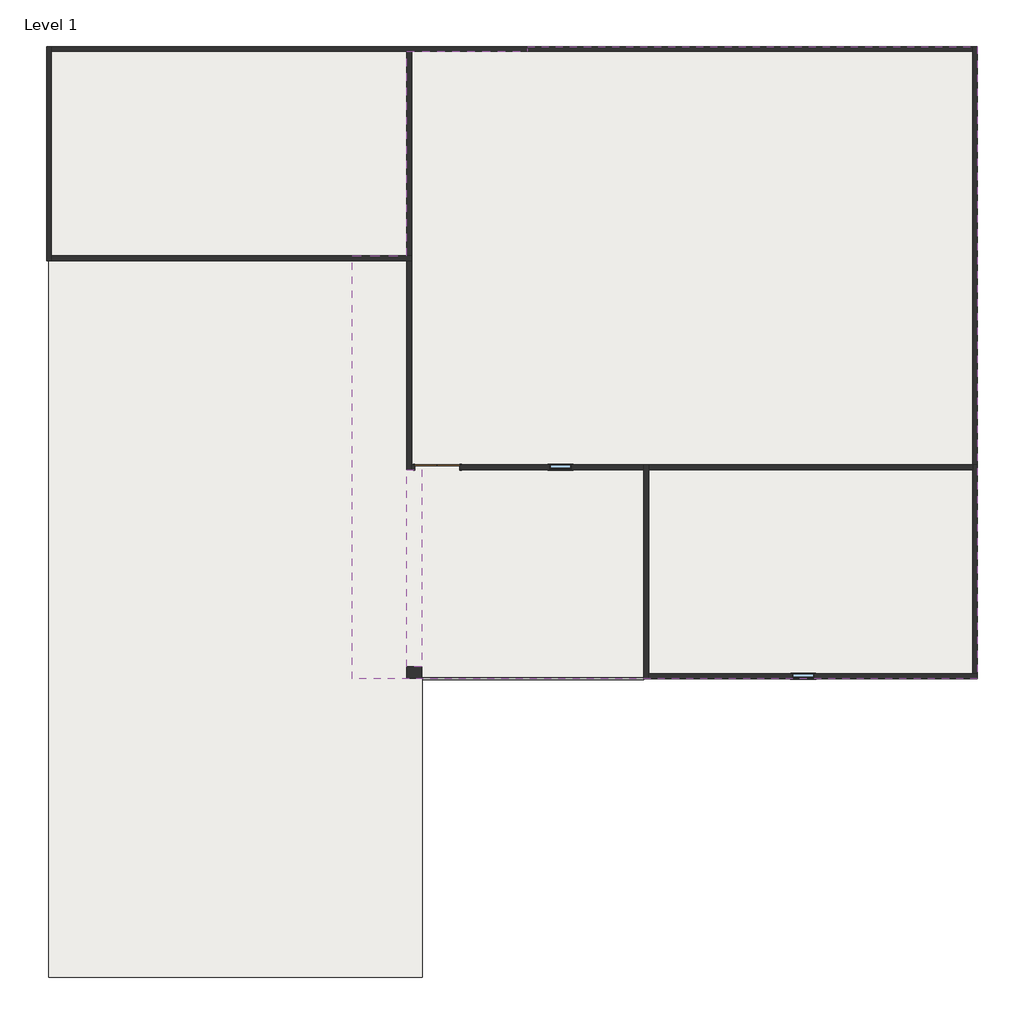
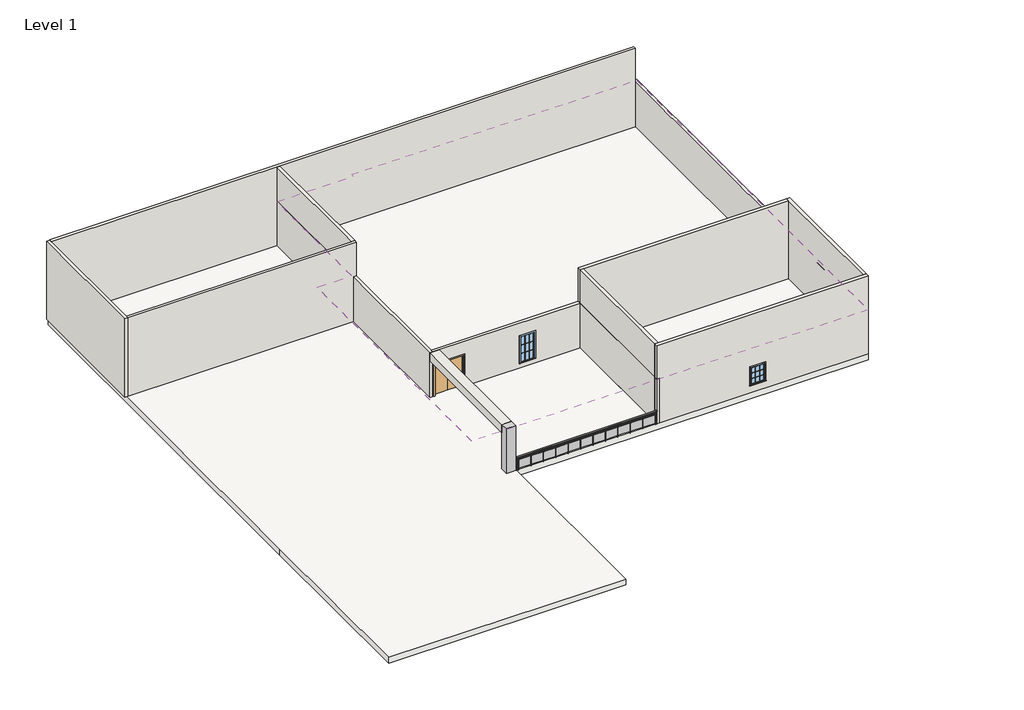
# One storey, incomplete: 13 walls, 2 windows, 1 column, 1 covering, 1 door, 1 railing, 1 slab.
"""IFC4 building model written with IfcOpenShell, lengths in millimetres."""

from ifc_helpers import new_model, si_unit, point, frame, origin, place, context, project, spatial, polyline, ellipse_curve, trimmed, outline, extrude, faceted_brep, transform, mapped, element, save
from ifc_brep_helpers import plane_surface, extruded_surface, advanced_brep
from components import m_rectangular_column_475_x_610mm_d36e7488, door_db0c0681, walls_1_walls_1_bd393664, window_ddc5d35f, window_0c844ac8

model = new_model("IFC4")

# Units and contexts
model_context = context("Model", 3, world=origin())
ifc_project = project(units=[si_unit("LENGTHUNIT", "METRE", prefix="MILLI")], contexts=[model_context])

# Site, building, storey
site = spatial("IfcSite", under=ifc_project)
building = spatial("IfcBuilding", under=site)
storey = spatial("IfcBuildingStorey", under=building, Name="Level 1", Elevation=3048.0)

# Column
placement = place(None, origin())
m_rectangular_column_475_x_610mm_shape = m_rectangular_column_475_x_610mm_d36e7488(model_context)
element("IfcColumn", 1, ObjectType="M_Rectangular Column : 475 x 610mm", at=placement, inside=storey, context=model_context, shape_type="MappedRepresentation", body=[
    mapped(m_rectangular_column_475_x_610mm_shape, transform((-2824.5479903, -9080.6874979, 0.0), x_axis=(1.0, 0.0, 0.0), y_axis=(0.0, 1.0, 0.0), z_axis=(0.0, 0.0, 1.0))),
])

# Covering
element("IfcCovering", 2, ObjectType="600 x 1200mm grid", at=placement, inside=storey, context=model_context, shape_type="SweptSolid", body=[
    extrude(outline(polyline([(-5354.6982739, -9333.0874979), (-5354.6982739, 7935.7125021), (-3125.3625081, 7935.7125021), (-3125.3625081, 16270.1125021), (1808.1017261, 16270.1125021), (1808.1017261, 16470.1125021), (20161.6374919, 16470.1125021), (20161.6374919, -9333.0874979), (-5354.6982739, -9333.0874979)]), holes=[polyline([(-4506.4859174, -9133.0874979), (6313.9140826, -9133.0874979), (6313.9140826, -7913.8874979), (-4506.4859174, -7913.8874979), (-4506.4859174, -9133.0874979)]), polyline([(-3051.6674392, 6921.3125021), (-4506.4859174, 6921.3125021), (-4506.4859174, -598.6874979), (-3051.6674392, -598.6874979), (-3051.6674392, 6921.3125021)])]), frame((0.0, 0.0, 6045.2), z_axis=(0.0, 0.0, 1.0), x_axis=(1.0, 0.0, 0.0)), (0.0, 0.0, 1.0), 52.0),
    extrude(outline(polyline([(-3473.1102813, -8081.6812121), (-3473.1102813, -8996.0812121), (-3549.3102813, -8996.0812121), (-3549.3102813, -8081.6812121), (-3473.1102813, -8081.6812121)])), frame((0.0, 0.0, 6045.2), z_axis=(0.0, 0.0, 1.0), x_axis=(1.0, 0.0, 0.0)), (0.0, 0.0, 1.0), 52.0),
    extrude(outline(polyline([(-2711.1102813, -8081.6812121), (-2711.1102813, -8996.0812121), (-2787.3102813, -8996.0812121), (-2787.3102813, -8081.6812121), (-2711.1102813, -8081.6812121)])), frame((0.0, 0.0, 6045.2), z_axis=(0.0, 0.0, 1.0), x_axis=(1.0, 0.0, 0.0)), (0.0, 0.0, 1.0), 52.0),
    extrude(outline(polyline([(-1771.3102813, -8081.6812121), (-1771.3102813, -8996.0812121), (-1847.5102813, -8996.0812121), (-1847.5102813, -8081.6812121), (-1771.3102813, -8081.6812121)])), frame((0.0, 0.0, 6045.2), z_axis=(0.0, 0.0, 1.0), x_axis=(1.0, 0.0, 0.0)), (0.0, 0.0, 1.0), 52.0),
    extrude(outline(polyline([(-856.9102813, -8081.6812121), (-856.9102813, -8996.0812121), (-933.1102813, -8996.0812121), (-933.1102813, -8081.6812121), (-856.9102813, -8081.6812121)])), frame((0.0, 0.0, 6045.2), z_axis=(0.0, 0.0, 1.0), x_axis=(1.0, 0.0, 0.0)), (0.0, 0.0, 1.0), 52.0),
    extrude(outline(polyline([(209.8897187, -8081.6812121), (209.8897187, -8996.0812121), (133.6897187, -8996.0812121), (133.6897187, -8081.6812121), (209.8897187, -8081.6812121)])), frame((0.0, 0.0, 6045.2), z_axis=(0.0, 0.0, 1.0), x_axis=(1.0, 0.0, 0.0)), (0.0, 0.0, 1.0), 52.0),
    extrude(outline(polyline([(1276.6897187, -8081.6812121), (1276.6897187, -8996.0812121), (1200.4897187, -8996.0812121), (1200.4897187, -8081.6812121), (1276.6897187, -8081.6812121)])), frame((0.0, 0.0, 6045.2), z_axis=(0.0, 0.0, 1.0), x_axis=(1.0, 0.0, 0.0)), (0.0, 0.0, 1.0), 52.0),
    extrude(outline(polyline([(2648.2897187, -8081.6812121), (2648.2897187, -8996.0812121), (2572.0897187, -8996.0812121), (2572.0897187, -8081.6812121), (2648.2897187, -8081.6812121)])), frame((0.0, 0.0, 6045.2), z_axis=(0.0, 0.0, 1.0), x_axis=(1.0, 0.0, 0.0)), (0.0, 0.0, 1.0), 52.0),
    extrude(outline(polyline([(4019.8897187, -8081.6812121), (4019.8897187, -8996.0812121), (3943.6897187, -8996.0812121), (3943.6897187, -8081.6812121), (4019.8897187, -8081.6812121)])), frame((0.0, 0.0, 6045.2), z_axis=(0.0, 0.0, 1.0), x_axis=(1.0, 0.0, 0.0)), (0.0, 0.0, 1.0), 52.0),
    extrude(outline(polyline([(5239.0897187, -8081.6812121), (5239.0897187, -8996.0812121), (5162.8897187, -8996.0812121), (5162.8897187, -8081.6812121), (5239.0897187, -8081.6812121)])), frame((0.0, 0.0, 6045.2), z_axis=(0.0, 0.0, 1.0), x_axis=(1.0, 0.0, 0.0)), (0.0, 0.0, 1.0), 52.0),
    extrude(outline(polyline([(-3153.2674392, 3237.4377462), (-3153.2674392, 2932.6377462), (-4423.2674392, 2932.6377462), (-4423.2674392, 3237.4377462), (-3153.2674392, 3237.4377462)])), frame((0.0, 0.0, 6045.2), z_axis=(0.0, 0.0, 1.0), x_axis=(1.0, 0.0, 0.0)), (0.0, 0.0, 1.0), 52.0),
    extrude(outline(polyline([(-3153.2674392, 5523.4377462), (-3153.2674392, 5218.6377462), (-4423.2674392, 5218.6377462), (-4423.2674392, 5523.4377462), (-3153.2674392, 5523.4377462)])), frame((0.0, 0.0, 6045.2), z_axis=(0.0, 0.0, 1.0), x_axis=(1.0, 0.0, 0.0)), (0.0, 0.0, 1.0), 52.0),
    extrude(outline(polyline([(-3153.2674392, 951.4377462), (-3153.2674392, 646.6377462), (-4423.2674392, 646.6377462), (-4423.2674392, 951.4377462), (-3153.2674392, 951.4377462)])), frame((0.0, 0.0, 6045.2), z_axis=(0.0, 0.0, 1.0), x_axis=(1.0, 0.0, 0.0)), (0.0, 0.0, 1.0), 52.0),
])

# Door
door_shape = door_db0c0681(model_context)
element("IfcDoor", 3, ObjectType="Door-Double-Flush_Panel : 72\" x 84\"", at=placement, inside=storey, context=model_context, shape_type="MappedRepresentation", body=[
    mapped(door_shape, transform((-1883.9625081, -698.6874979, 3048.0), x_axis=(1.0, 0.0, 0.0), y_axis=(0.0, 1.0, 0.0), z_axis=(0.0, 0.0, 1.0))),
])

# Railing
element("IfcRailing", 4, ObjectType="Glass Panel - Bottom Fill", at=placement, inside=storey, context=model_context, shape_type="SolidModel", body=[
    advanced_brep(
    [(-2473.5625081, -9293.6967328, 3948.0), (-2473.5625081, -9373.6967328, 3948.0), (6550.4374919, -9293.6967328, 3948.0), (6550.4374919, -9373.6967328, 3948.0)],
    [
        (0, 1, ellipse_curve(frame((-2473.5625081, -9333.6967328, 3948.0), z_axis=(-1.0, 0.0, 0.0), x_axis=(0.0, -1.0, 0.0)), 40.0, 30.0)),
        (1, 0, ellipse_curve(frame((-2473.5625081, -9333.6967328, 3948.0), z_axis=(-1.0, 0.0, 0.0), x_axis=(0.0, -1.0, 0.0)), 40.0, 30.0)),
        (2, 3, ellipse_curve(frame((6550.4374919, -9333.6967328, 3948.0), z_axis=(1.0, 0.0, 0.0), x_axis=(0.0, -1.0, 0.0)), 40.0, 30.0)),
        (3, 2, ellipse_curve(frame((6550.4374919, -9333.6967328, 3948.0), z_axis=(1.0, 0.0, 0.0), x_axis=(0.0, -1.0, 0.0)), 40.0, 30.0)),
        (1, 3),
        (2, 0),
    ],
    [
        plane_surface(frame((-2473.5625081, -9333.6967328, 3948.0), z_axis=(-1.0, 0.0, 0.0), x_axis=(0.0, 1.0, 0.0))),
        plane_surface(frame((6550.4374919, -9333.6967328, 3948.0), z_axis=(1.0, 0.0, 0.0), x_axis=(0.0, 1.0, 0.0))),
        extruded_surface(trimmed(ellipse_curve(frame((6550.4374919, -9333.6967328, 3948.0), z_axis=(-1.0, 0.0, 0.0), x_axis=(0.0, -1.0, 0.0)), 40.0, 30.0), [point((6550.4374919, -9373.6967328, 3948.0))], [point((6550.4374919, -9293.6967328, 3948.0))], True, "CARTESIAN"), (-9024.0, 0.0, 0.0), 9024.0),
        extruded_surface(trimmed(ellipse_curve(frame((6550.4374919, -9333.6967328, 3948.0), z_axis=(-1.0, 0.0, 0.0), x_axis=(0.0, -1.0, 0.0)), 40.0, 30.0), [point((6550.4374919, -9293.6967328, 3948.0))], [point((6550.4374919, -9373.6967328, 3948.0))], True, "CARTESIAN"), (-9024.0, 0.0, 0.0), 9024.0),
    ],
    [
        (0, [[1, 2]]),
        (1, [[3, 4]]),
        (2, [[-2, 5, -3, 6]]),
        (3, [[-1, -6, -4, -5]]),
    ],
),
    extrude(outline(polyline([(-2473.5625081, -9343.0874979), (-2473.5625081, -9323.0874979), (6550.4374919, -9323.0874979), (6550.4374919, -9343.0874979), (-2473.5625081, -9343.0874979)])), frame((0.0, 0.0, 3828.0), z_axis=(0.0, 0.0, 1.0), x_axis=(1.0, 0.0, 0.0)), (0.0, 0.0, 1.0), 20.0),
    extrude(outline(polyline([(-2473.5625081, -9343.0874979), (-2473.5625081, -9323.0874979), (6550.4374919, -9323.0874979), (6550.4374919, -9343.0874979), (-2473.5625081, -9343.0874979)])), frame((0.0, 0.0, 3728.0), z_axis=(0.0, 0.0, 1.0), x_axis=(1.0, 0.0, 0.0)), (0.0, 0.0, 1.0), 20.0),
    extrude(outline(polyline([(6432.4374919, -9308.0874979), (6444.4374919, -9308.0874979), (6444.4374919, -9358.0874979), (6432.4374919, -9358.0874979), (6432.4374919, -9308.0874979)])), frame((0.0, 0.0, 3048.0), z_axis=(0.0, 0.0, 1.0), x_axis=(1.0, 0.0, 0.0)), (0.0, 0.0, 1.0), 869.8465326),
    extrude(outline(polyline([(5638.4374919, -9334.812308), (6438.4374919, -9334.812308), (6438.4374919, -9339.812308), (5638.4374919, -9339.812308), (5638.4374919, -9334.812308)])), frame((0.0, 0.0, 3148.0), z_axis=(0.0, 0.0, 1.0), x_axis=(1.0, 0.0, 0.0)), (0.0, 0.0, 1.0), 580.0),
    extrude(outline(polyline([(5632.4374919, -9308.0874979), (5644.4374919, -9308.0874979), (5644.4374919, -9358.0874979), (5632.4374919, -9358.0874979), (5632.4374919, -9308.0874979)])), frame((0.0, 0.0, 3048.0), z_axis=(0.0, 0.0, 1.0), x_axis=(1.0, 0.0, 0.0)), (0.0, 0.0, 1.0), 869.8465326),
    extrude(outline(polyline([(4838.4374919, -9334.812308), (5638.4374919, -9334.812308), (5638.4374919, -9339.812308), (4838.4374919, -9339.812308), (4838.4374919, -9334.812308)])), frame((0.0, 0.0, 3148.0), z_axis=(0.0, 0.0, 1.0), x_axis=(1.0, 0.0, 0.0)), (0.0, 0.0, 1.0), 580.0),
    extrude(outline(polyline([(4832.4374919, -9308.0874979), (4844.4374919, -9308.0874979), (4844.4374919, -9358.0874979), (4832.4374919, -9358.0874979), (4832.4374919, -9308.0874979)])), frame((0.0, 0.0, 3048.0), z_axis=(0.0, 0.0, 1.0), x_axis=(1.0, 0.0, 0.0)), (0.0, 0.0, 1.0), 869.8465326),
    extrude(outline(polyline([(4038.4374919, -9334.812308), (4838.4374919, -9334.812308), (4838.4374919, -9339.812308), (4038.4374919, -9339.812308), (4038.4374919, -9334.812308)])), frame((0.0, 0.0, 3148.0), z_axis=(0.0, 0.0, 1.0), x_axis=(1.0, 0.0, 0.0)), (0.0, 0.0, 1.0), 580.0),
    extrude(outline(polyline([(4032.4374919, -9308.0874979), (4044.4374919, -9308.0874979), (4044.4374919, -9358.0874979), (4032.4374919, -9358.0874979), (4032.4374919, -9308.0874979)])), frame((0.0, 0.0, 3048.0), z_axis=(0.0, 0.0, 1.0), x_axis=(1.0, 0.0, 0.0)), (0.0, 0.0, 1.0), 869.8465326),
    extrude(outline(polyline([(3238.4374919, -9334.812308), (4038.4374919, -9334.812308), (4038.4374919, -9339.812308), (3238.4374919, -9339.812308), (3238.4374919, -9334.812308)])), frame((0.0, 0.0, 3148.0), z_axis=(0.0, 0.0, 1.0), x_axis=(1.0, 0.0, 0.0)), (0.0, 0.0, 1.0), 580.0),
    extrude(outline(polyline([(3232.4374919, -9308.0874979), (3244.4374919, -9308.0874979), (3244.4374919, -9358.0874979), (3232.4374919, -9358.0874979), (3232.4374919, -9308.0874979)])), frame((0.0, 0.0, 3048.0), z_axis=(0.0, 0.0, 1.0), x_axis=(1.0, 0.0, 0.0)), (0.0, 0.0, 1.0), 869.8465326),
    extrude(outline(polyline([(2438.4374919, -9334.812308), (3238.4374919, -9334.812308), (3238.4374919, -9339.812308), (2438.4374919, -9339.812308), (2438.4374919, -9334.812308)])), frame((0.0, 0.0, 3148.0), z_axis=(0.0, 0.0, 1.0), x_axis=(1.0, 0.0, 0.0)), (0.0, 0.0, 1.0), 580.0),
    extrude(outline(polyline([(2432.4374919, -9308.0874979), (2444.4374919, -9308.0874979), (2444.4374919, -9358.0874979), (2432.4374919, -9358.0874979), (2432.4374919, -9308.0874979)])), frame((0.0, 0.0, 3048.0), z_axis=(0.0, 0.0, 1.0), x_axis=(1.0, 0.0, 0.0)), (0.0, 0.0, 1.0), 869.8465326),
    extrude(outline(polyline([(1638.4374919, -9334.812308), (2438.4374919, -9334.812308), (2438.4374919, -9339.812308), (1638.4374919, -9339.812308), (1638.4374919, -9334.812308)])), frame((0.0, 0.0, 3148.0), z_axis=(0.0, 0.0, 1.0), x_axis=(1.0, 0.0, 0.0)), (0.0, 0.0, 1.0), 580.0),
    extrude(outline(polyline([(1632.4374919, -9308.0874979), (1644.4374919, -9308.0874979), (1644.4374919, -9358.0874979), (1632.4374919, -9358.0874979), (1632.4374919, -9308.0874979)])), frame((0.0, 0.0, 3048.0), z_axis=(0.0, 0.0, 1.0), x_axis=(1.0, 0.0, 0.0)), (0.0, 0.0, 1.0), 869.8465326),
    extrude(outline(polyline([(838.4374919, -9334.812308), (1638.4374919, -9334.812308), (1638.4374919, -9339.812308), (838.4374919, -9339.812308), (838.4374919, -9334.812308)])), frame((0.0, 0.0, 3148.0), z_axis=(0.0, 0.0, 1.0), x_axis=(1.0, 0.0, 0.0)), (0.0, 0.0, 1.0), 580.0),
    extrude(outline(polyline([(832.4374919, -9308.0874979), (844.4374919, -9308.0874979), (844.4374919, -9358.0874979), (832.4374919, -9358.0874979), (832.4374919, -9308.0874979)])), frame((0.0, 0.0, 3048.0), z_axis=(0.0, 0.0, 1.0), x_axis=(1.0, 0.0, 0.0)), (0.0, 0.0, 1.0), 869.8465326),
    extrude(outline(polyline([(38.4374919, -9334.812308), (838.4374919, -9334.812308), (838.4374919, -9339.812308), (38.4374919, -9339.812308), (38.4374919, -9334.812308)])), frame((0.0, 0.0, 3148.0), z_axis=(0.0, 0.0, 1.0), x_axis=(1.0, 0.0, 0.0)), (0.0, 0.0, 1.0), 580.0),
    extrude(outline(polyline([(32.4374919, -9308.0874979), (44.4374919, -9308.0874979), (44.4374919, -9358.0874979), (32.4374919, -9358.0874979), (32.4374919, -9308.0874979)])), frame((0.0, 0.0, 3048.0), z_axis=(0.0, 0.0, 1.0), x_axis=(1.0, 0.0, 0.0)), (0.0, 0.0, 1.0), 869.8465326),
    extrude(outline(polyline([(-761.5625081, -9334.812308), (38.4374919, -9334.812308), (38.4374919, -9339.812308), (-761.5625081, -9339.812308), (-761.5625081, -9334.812308)])), frame((0.0, 0.0, 3148.0), z_axis=(0.0, 0.0, 1.0), x_axis=(1.0, 0.0, 0.0)), (0.0, 0.0, 1.0), 580.0),
    extrude(outline(polyline([(-767.5625081, -9308.0874979), (-755.5625081, -9308.0874979), (-755.5625081, -9358.0874979), (-767.5625081, -9358.0874979), (-767.5625081, -9308.0874979)])), frame((0.0, 0.0, 3048.0), z_axis=(0.0, 0.0, 1.0), x_axis=(1.0, 0.0, 0.0)), (0.0, 0.0, 1.0), 869.8465326),
    extrude(outline(polyline([(-1561.5625081, -9334.812308), (-761.5625081, -9334.812308), (-761.5625081, -9339.812308), (-1561.5625081, -9339.812308), (-1561.5625081, -9334.812308)])), frame((0.0, 0.0, 3148.0), z_axis=(0.0, 0.0, 1.0), x_axis=(1.0, 0.0, 0.0)), (0.0, 0.0, 1.0), 580.0),
    extrude(outline(polyline([(-1567.5625081, -9308.0874979), (-1555.5625081, -9308.0874979), (-1555.5625081, -9358.0874979), (-1567.5625081, -9358.0874979), (-1567.5625081, -9308.0874979)])), frame((0.0, 0.0, 3048.0), z_axis=(0.0, 0.0, 1.0), x_axis=(1.0, 0.0, 0.0)), (0.0, 0.0, 1.0), 869.8465326),
    extrude(outline(polyline([(-2361.5625081, -9334.812308), (-1561.5625081, -9334.812308), (-1561.5625081, -9339.812308), (-2361.5625081, -9339.812308), (-2361.5625081, -9334.812308)])), frame((0.0, 0.0, 3148.0), z_axis=(0.0, 0.0, 1.0), x_axis=(1.0, 0.0, 0.0)), (0.0, 0.0, 1.0), 580.0),
    extrude(outline(polyline([(-2367.5625081, -9308.0874979), (-2355.5625081, -9308.0874979), (-2355.5625081, -9358.0874979), (-2367.5625081, -9358.0874979), (-2367.5625081, -9308.0874979)])), frame((0.0, 0.0, 3048.0), z_axis=(0.0, 0.0, 1.0), x_axis=(1.0, 0.0, 0.0)), (0.0, 0.0, 1.0), 869.8465326),
    extrude(outline(polyline([(6542.4374919, -9308.0874979), (6554.4374919, -9308.0874979), (6554.4374919, -9358.0874979), (6542.4374919, -9358.0874979), (6542.4374919, -9308.0874979)])), frame((0.0, 0.0, 3048.0), z_axis=(0.0, 0.0, 1.0), x_axis=(1.0, 0.0, 0.0)), (0.0, 0.0, 1.0), 869.8465326),
    extrude(outline(polyline([(-2477.5625081, -9308.0874979), (-2465.5625081, -9308.0874979), (-2465.5625081, -9358.0874979), (-2477.5625081, -9358.0874979), (-2477.5625081, -9308.0874979)])), frame((0.0, 0.0, 3048.0), z_axis=(0.0, 0.0, 1.0), x_axis=(1.0, 0.0, 0.0)), (0.0, 0.0, 1.0), 869.8465326),
])

# Slab
element("IfcSlab", 5, ObjectType="Generic Floor - 400mm", at=placement, inside=storey, context=model_context, shape_type="SweptSolid", body=[
    extrude(outline(polyline([(20161.6374919, 16470.1125021), (20161.6374919, -9333.0874979), (-2493.5625081, -9333.0874979), (-2493.5625081, -21525.0874979), (-17733.5625081, -21525.0874979), (-17733.5625081, -9333.0874979), (-17733.5625081, 16470.1125021), (20161.6374919, 16470.1125021)])), frame((0.0, 0.0, 2648.0), z_axis=(0.0, 0.0, 1.0), x_axis=(1.0, 0.0, 0.0)), (0.0, 0.0, 1.0), 400.0),
])

# Walls
element("IfcWall", 6, ObjectType="Generic - 9\"", at=placement, inside=storey, context=model_context, shape_type="Brep", body=[
    faceted_brep([(-17633.5625081, 16270.1125021, 3048.0), (-3125.3625081, 16270.1125021, 3048.0), (-2925.3625081, 16270.1125021, 3048.0), (19961.6374919, 16270.1125021, 3048.0), (19961.6374919, 16270.1125021, 8393.9849899), (-17633.5625081, 16270.1125021, 8393.9849899), (-17633.5625081, 16470.1125021, 3048.0), (-17633.5625081, 16470.1125021, 8382.0), (-17633.5625081, 16470.1125021, 8393.9849899), (19961.6374919, 16470.1125021, 8393.9849899), (19961.6374919, 16470.1125021, 6096.0), (19961.6374919, 16470.1125021, 3048.0)], [[[0, 1, 2, 3, 4, 5]], [[6, 7, 8, 9, 10, 11]], [[3, 2, 1, 0, 6, 11]], [[5, 4, 9, 8]], [[4, 3, 11, 10, 9]], [[0, 5, 8, 7, 6]]]),
])
element("IfcWall", 7, ObjectType="Generic - 9\"", at=placement, inside=storey, context=model_context, shape_type="Brep", body=[
    faceted_brep([(-2925.3625081, -798.6874979, 3048.0), (-2925.3625081, -598.6874979, 3048.0), (-2925.3625081, 16270.1125021, 3048.0), (-2925.3625081, 16270.1125021, 6096.0), (-2925.3625081, -598.6874979, 6096.0), (-2925.3625081, -798.6874979, 6096.0), (-3125.3625081, -798.6874979, 3048.0), (-3125.3625081, -798.6874979, 6096.0), (-3125.3625081, 16270.1125021, 6096.0), (-3125.3625081, 16270.1125021, 3048.0)], [[[0, 1, 2, 3, 4, 5]], [[6, 7, 8, 9]], [[3, 2, 9, 8]], [[0, 5, 7, 6]], [[2, 1, 0, 6, 9]], [[5, 4, 3, 8, 7]]]),
])
element("IfcWall", 8, ObjectType="Generic - 9\"", at=placement, inside=storey, context=model_context, shape_type="Brep", body=[
    faceted_brep([(20161.6374919, -9133.0874979, 8382.0), (20161.6374919, -9133.0874979, 6096.0), (20161.6374919, -9133.0874979, 3048.0), (19961.6374919, -9133.0874979, 3048.0), (6750.4374919, -9133.0874979, 3048.0), (6750.4374919, -9133.0874979, 6096.0), (6550.4374919, -9133.0874979, 6096.0), (6550.4374919, -9133.0874979, 8382.0), (6750.4374919, -9133.0874979, 8382.0), (19961.6374919, -9133.0874979, 8382.0), (12594.0374919, -9133.0874979, 4772.8031675), (12594.0374919, -9133.0874979, 3553.6031675), (13508.4374919, -9133.0874979, 3553.6031675), (13508.4374919, -9133.0874979, 4772.8031675), (20161.6374919, -9333.0874979, 3048.0), (20161.6374919, -9333.0874979, 8382.0), (6550.4374919, -9333.0874979, 8382.0), (6550.4374919, -9333.0874979, 6096.0), (6750.4374919, -9333.0874979, 6096.0), (6750.4374919, -9333.0874979, 3048.0), (12594.0374919, -9333.0874979, 4772.8031675), (13508.4374919, -9333.0874979, 4772.8031675), (13508.4374919, -9333.0874979, 3553.6031675), (12594.0374919, -9333.0874979, 3553.6031675)], [[[0, 1, 2, 3, 4, 5, 6, 7, 8, 9], [10, 11, 12, 13]], [[14, 15, 16, 17, 18, 19], [20, 21, 22, 23]], [[4, 3, 2, 14, 19]], [[0, 9, 8, 7, 16, 15]], [[0, 15, 14, 2, 1]], [[17, 6, 5, 18]], [[5, 4, 19, 18]], [[7, 6, 17, 16]], [[11, 10, 20, 23]], [[12, 11, 23, 22]], [[13, 12, 22, 21]], [[10, 13, 21, 20]]]),
])
element("IfcWall", 9, ObjectType="Generic - 9\"", at=placement, inside=storey, context=model_context, shape_type="Brep", body=[
    faceted_brep([(19961.6374919, 16470.1125021, 3048.0), (19961.6374919, 16270.1125021, 3048.0), (19961.6374919, -9133.0874979, 3048.0), (19961.6374919, -9133.0874979, 6096.0), (19961.6374919, 16470.1125021, 6096.0), (20161.6374919, 16470.1125021, 3048.0), (20161.6374919, 16470.1125021, 6096.0), (20161.6374919, -9133.0874979, 6096.0), (20161.6374919, -9133.0874979, 3048.0)], [[[0, 1, 2, 3, 4]], [[5, 6, 7, 8]], [[2, 1, 0, 5, 8]], [[4, 3, 7, 6]], [[0, 4, 6, 5]], [[3, 2, 8, 7]]]),
])
element("IfcWall", 10, ObjectType="Generic - 9\"", at=placement, inside=storey, context=model_context, shape_type="Brep", body=[
    faceted_brep([(6750.4374919, -9333.0874979, 3048.0), (6750.4374919, -9133.0874979, 3048.0), (6750.4374919, -798.6874979, 3048.0), (6750.4374919, -598.6874979, 3048.0), (6750.4374919, -598.6874979, 6096.0), (6750.4374919, -798.6874979, 6096.0), (6750.4374919, -9133.0874979, 6096.0), (6750.4374919, -9333.0874979, 6096.0), (6550.4374919, -9333.0874979, 3048.0), (6550.4374919, -9333.0874979, 6096.0), (6550.4374919, -9133.0874979, 6096.0), (6550.4374919, -798.6874979, 6096.0), (6550.4374919, -598.6874979, 6096.0), (6550.4374919, -598.6874979, 3048.0), (6550.4374919, -798.6874979, 3048.0)], [[[0, 1, 2, 3, 4, 5, 6, 7]], [[8, 9, 10, 11, 12, 13, 14]], [[3, 2, 1, 0, 8, 14, 13]], [[7, 6, 5, 4, 12, 11, 10, 9]], [[0, 7, 9, 8]], [[4, 3, 13, 12]]]),
])
element("IfcWall", 11, ObjectType="Generic - 9\"", at=placement, inside=storey, context=model_context, shape_type="SweptSolid", body=[
    extrude(outline(polyline([(6096.0, 6550.4374919), (6096.0, -2925.3625081), (3048.0, -2925.3625081), (3048.0, -2798.3625081), (5181.6, -2798.3625081), (5181.6, -969.5625081), (3048.0, -969.5625081), (3048.0, 6550.4374919), (6096.0, 6550.4374919)]), holes=[polyline([(5181.6, 2688.0374919), (5181.6, 3602.4374919), (3352.8, 3602.4374919), (3352.8, 2688.0374919), (5181.6, 2688.0374919)])]), frame((0.0, -798.6874979, 0.0), z_axis=(0.0, 1.0, 0.0), x_axis=(0.0, 0.0, 1.0)), (0.0, 0.0, 1.0), 200.0),
])
element("IfcWall", 12, ObjectType="Generic - 9\"", at=placement, inside=storey, context=model_context, shape_type="Brep", body=[
    faceted_brep([(-17633.5625081, 7735.7125021, 3048.0), (-17633.5625081, 7935.7125021, 3048.0), (-17633.5625081, 16270.1125021, 3048.0), (-17633.5625081, 16470.1125021, 3048.0), (-17633.5625081, 16470.1125021, 8382.0), (-17633.5625081, 7935.7125021, 8382.0), (-17633.5625081, 7735.7125021, 8382.0), (-17833.5625081, 7735.7125021, 3048.0), (-17833.5625081, 7735.7125021, 8382.0), (-17833.5625081, 16470.1125021, 8382.0), (-17833.5625081, 16470.1125021, 3048.0)], [[[0, 1, 2, 3, 4, 5, 6]], [[7, 8, 9, 10]], [[3, 2, 1, 0, 7, 10]], [[6, 5, 4, 9, 8]], [[0, 6, 8, 7]], [[4, 3, 10, 9]]]),
])
element("IfcWall", 13, ObjectType="Generic - 9\"", at=placement, inside=storey, context=model_context, shape_type="Brep", body=[
    faceted_brep([(-2925.3625081, 7935.7125021, 8382.0), (-2925.3625081, 7935.7125021, 3048.0), (-3125.3625081, 7935.7125021, 3048.0), (-17633.5625081, 7935.7125021, 3048.0), (-17633.5625081, 7935.7125021, 8382.0), (-3125.3625081, 7935.7125021, 8382.0), (-2925.3625081, 7735.7125021, 3048.0), (-2925.3625081, 7735.7125021, 6096.0), (-2925.3625081, 7735.7125021, 8382.0), (-3125.3625081, 7735.7125021, 8382.0), (-17633.5625081, 7735.7125021, 8382.0), (-17633.5625081, 7735.7125021, 3048.0)], [[[0, 1, 2, 3, 4, 5]], [[6, 7, 8, 9, 10, 11]], [[4, 3, 11, 10]], [[3, 2, 1, 6, 11]], [[0, 5, 4, 10, 9, 8]], [[0, 8, 7, 6, 1]]]),
])
element("IfcWall", 14, ObjectType="Generic - 9\"", at=placement, inside=storey, context=model_context, shape_type="SweptSolid", body=[
    extrude(outline(polyline([(-3125.3625081, 7935.7125021), (-3125.3625081, 16270.1125021), (-2925.3625081, 16270.1125021), (-2925.3625081, 7935.7125021), (-3125.3625081, 7935.7125021)])), frame((0.0, 0.0, 3048.0), z_axis=(0.0, 0.0, 1.0), x_axis=(1.0, 0.0, 0.0)), (0.0, 0.0, 1.0), 5334.0),
])
element("IfcWall", 15, ObjectType="Generic - 9\"", at=placement, inside=storey, context=model_context, shape_type="Brep", body=[
    faceted_brep([(19961.6374919, -598.6874979, 3048.0), (19961.6374919, -798.6874979, 3048.0), (19961.6374919, -9133.0874979, 3048.0), (19961.6374919, -9133.0874979, 8382.0), (19961.6374919, -798.6874979, 8382.0), (19961.6374919, -598.6874979, 8382.0), (20161.6374919, -598.6874979, 3048.0), (20161.6374919, -598.6874979, 8382.0), (20161.6374919, -9133.0874979, 8382.0), (20161.6374919, -9133.0874979, 3048.0)], [[[0, 1, 2, 3, 4, 5]], [[6, 7, 8, 9]], [[2, 1, 0, 6, 9]], [[5, 4, 3, 8, 7]], [[0, 5, 7, 6]], [[2, 9, 8, 3]]]),
])
element("IfcWall", 16, ObjectType="Generic - 9\"", at=placement, inside=storey, context=model_context, shape_type="Brep", body=[
    faceted_brep([(6750.4374919, -798.6874979, 3048.0), (19961.6374919, -798.6874979, 3048.0), (19961.6374919, -798.6874979, 8382.0), (6750.4374919, -798.6874979, 8382.0), (6550.4374919, -798.6874979, 8382.0), (6550.4374919, -798.6874979, 7315.2), (6550.4374919, -798.6874979, 6096.0), (6750.4374919, -798.6874979, 6096.0), (6750.4374919, -598.6874979, 3048.0), (6750.4374919, -598.6874979, 6096.0), (6550.4374919, -598.6874979, 6096.0), (6550.4374919, -598.6874979, 7315.2), (6550.4374919, -598.6874979, 8382.0), (19961.6374919, -598.6874979, 8382.0), (19961.6374919, -598.6874979, 3048.0)], [[[0, 1, 2, 3, 4, 5, 6, 7]], [[8, 9, 10, 11, 12, 13, 14]], [[1, 0, 8, 14]], [[4, 3, 2, 13, 12]], [[2, 1, 14, 13]], [[6, 10, 9, 7]], [[0, 7, 9, 8]], [[4, 12, 11, 10, 6, 5]]]),
])
element("IfcWall", 17, ObjectType="Generic - 9\"", at=placement, inside=storey, context=model_context, shape_type="Brep", body=[
    faceted_brep([(6750.4374919, -9133.0874979, 8382.0), (6750.4374919, -9133.0874979, 3048.0), (6750.4374919, -798.6874979, 3048.0), (6750.4374919, -798.6874979, 8382.0), (6550.4374919, -9133.0874979, 3048.0), (6550.4374919, -9133.0874979, 6096.0), (6550.4374919, -9133.0874979, 8382.0), (6550.4374919, -798.6874979, 8382.0), (6550.4374919, -798.6874979, 6096.0), (6550.4374919, -798.6874979, 3048.0)], [[[0, 1, 2, 3]], [[4, 5, 6, 7, 8, 9]], [[2, 1, 4, 9]], [[0, 3, 7, 6]], [[0, 6, 5, 4, 1]], [[2, 9, 8, 7, 3]]]),
])
walls_1_walls_1_shape = walls_1_walls_1_bd393664(model_context)
element("IfcWall", 18, ObjectType="Walls 1 : Walls 1", at=placement, inside=storey, context=model_context, shape_type="MappedRepresentation", body=[
    mapped(walls_1_walls_1_shape, transform((0.0, 0.0, 0.0), x_axis=(1.0, 0.0, 0.0), y_axis=(0.0, 1.0, 0.0), z_axis=(0.0, 0.0, 1.0))),
])

# Windows
window_shape = window_ddc5d35f(model_context)
element("IfcWindow", 19, ObjectType="Casement 3x3 with Trim : 36\" x 48\"", at=placement, inside=storey, context=model_context, shape_type="MappedRepresentation", body=[
    mapped(window_shape, transform((13051.2374919, -9233.0874979, 2639.2031675), x_axis=(-1.0, 0.0, 0.0), y_axis=(0.0, -1.0, 0.0), z_axis=(0.0, 0.0, 1.0))),
])
window_2_shape = window_0c844ac8(model_context)
element("IfcWindow", 20, ObjectType="Casement 3x3 with Trim : 36\" x 72\"", at=placement, inside=storey, context=model_context, shape_type="MappedRepresentation", body=[
    mapped(window_2_shape, transform((3145.2374919, -698.6874979, 3048.0), x_axis=(-1.0, 0.0, 0.0), y_axis=(0.0, -1.0, 0.0), z_axis=(0.0, 0.0, 1.0))),
])

save(model, "model.ifc")

# Revit data of these elements
# Type "M_Rectangular Column : 475 x 610mm"
#   Depth = 1' - 6.70079"
#   Offset Base = 0' - 0"
#   Offset Top = 0' - 0"
#   Width = 2' - 0.01575"
#   Material = none
# Type "600 x 1200mm grid"
#   built-in parameter 1002203 = 1 (stored number, unit not read)
#   built-in parameter 1002202 = 1 (stored number, unit not read)
#   Layers, outside or top first: 0' - 1.41732" "Default" (function 1); 0' - 0.62992" "Ceiling Tile 600 x 1200" (function 5)
# Type "Door-Double-Flush_Panel : 72\" x 84\""
#   Type Mark = "22"
#   Construction Type Id = "DOOR"
#   Assembly Code = "C1020"
#   Analytic Construction = "Wooden"
#   Thickness = 0' - 2"
#   Thermal Resistance (R) = 0.455703 (m²·K)/W
#   Swing Angle [instance default] = 90.00°
#   Panel Width = 3' - 0"
#   Heat Transfer Coefficient (U) = 2.19465 W/(m²·K)
#   Height = 7' - 0"
#   Trim Projection Ext = 0' - 1"
#   Trim Projection Int = 0' - 1"
#   Trim Width = 0' - 3"
#   Width = 6' - 0"
#   Define Thermal Properties by = 1
#   Panel Material = Wood - Birch - Solid Stained Light Low Gloss
#   Trim Material = Paint - Sienna
#   Visual Light Transmittance = 0
#   Solar Heat Gain Coefficient = 0
#   Function = (empty or 0)
#   Wall Closure = (empty or 0)
# Type "Glass Panel - Bottom Fill"
#   built-in parameter 1008612 = 0.019685 (stored number, unit not read)
#   built-in parameter 1008611 = 0.019685 (stored number, unit not read)
#   built-in parameter 1008609 = 0.902231 (stored number, unit not read)
#   built-in parameter 1008604 = 0.19685 (stored number, unit not read)
#   built-in parameter 1008603 = 0.164042 (stored number, unit not read)
#   Railing Height = 2' - 11.43307"
#   built-in parameter 1008630 = 2
#   built-in parameter 1008610 = 2
# Type "Generic Floor - 400mm"
#   Function = 0
#   Layers, outside or top first: 1' - 3.74803" no material (function 1)
# Type "Generic - 9\""
#   Layers, outside or top first: 0' - 7.87402" no material (function 1)
# Type "Casement 3x3 with Trim : 36\" x 48\""
#   Type Mark = "19"
#   Construction Type Id = "GSP4R"
#   Assembly Code = "B2020100"
#   Analytic Construction = "1/8 in Pilkington single glazing"
#   Visual Light Transmittance = 0.9
#   Solar Heat Gain Coefficient = 0.78
#   Heat Transfer Coefficient (U) = 3.6886 W/(m²·K)
#   Height = 4' - 0"
#   Default Sill Height = 3' - 0"
#   Trim Projection - Ext. = 0' - 0 1/2"
#   Trim Projection - Int. = 0' - 0 3/4"
#   Trim Width - Exterior = 0' - 3 1/2"
#   Trim Width - Interior = 0' - 3 1/2"
#   Width = 3' - 0"
#   Window Inset = 0' - 0 3/4"
#   Define Thermal Properties by = 1
#   Glass Pane Material = Glass
#   Sash Material = Sash
#   Trim Exterior Material = Trim
#   Trim Interior Material = Trim
#   Wall Closure = (empty or 0)
# Type "Casement 3x3 with Trim : 36\" x 72\""
#   Type Mark = "21"
#   Construction Type Id = "GSP4R"
#   Assembly Code = "B2020100"
#   Analytic Construction = "1/8 in Pilkington single glazing"
#   Visual Light Transmittance = 0.9
#   Solar Heat Gain Coefficient = 0.78
#   Heat Transfer Coefficient (U) = 3.6886 W/(m²·K)
#   Height = 6' - 0"
#   Default Sill Height = 1' - 0"
#   Trim Projection - Ext. = 0' - 0 1/2"
#   Trim Projection - Int. = 0' - 0 3/4"
#   Trim Width - Exterior = 0' - 3 1/2"
#   Trim Width - Interior = 0' - 3 1/2"
#   Width = 3' - 0"
#   Window Inset = 0' - 0 3/4"
#   Define Thermal Properties by = 1
#   Glass Pane Material = Glass
#   Sash Material = Sash
#   Trim Exterior Material = Trim
#   Trim Interior Material = Trim
#   Wall Closure = (empty or 0)
# Element 1 (IfcColumn, "M_Rectangular Column : 475 x 610mm")
#   Phase Created = New Construction
# Element 2 (IfcCovering, "600 x 1200mm grid")
#   Height Offset From Level = 9' - 10"
#   Phase Created = New Construction
#   Materials on its faces: "Ceiling Tile 600 x 1200", "Default"
# Element 3 (IfcDoor, "Door-Double-Flush_Panel : 72\" x 84\"")
#   Swing Angle = 90.00°
#   Phase Created = New Construction
#   Materials on its faces: "Paint - Sienna", "Wood - Birch - Solid Stained Light Low Gloss"
# Element 4 (IfcRailing, "Glass Panel - Bottom Fill")
#   Phase Created = New Construction
#   Materials on its faces: "Metal - Stainless Steel,Polished", "Glass"
# Element 5 (IfcSlab, "Generic Floor - 400mm")
#   Height Offset From Level = 0' - 0"
#   Phase Created = New Construction
#   Materials on its faces: "Default Roof"
# Element 6 (IfcWall, "Generic - 9\"")
#   Top Offset = 0' - 0"
#   Base Offset = 0' - 0"
#   Unconnected Height = 17' - 6.47185"
#   wall height = 17' - 6.47185"
#   Phase Created = New Construction
#   Base Constraint = Level 1
#   Materials on its faces: "Default Wall"
# Elements 7, 9, 10, 11 (IfcWall, "Generic - 9\"")
#   Top Offset = 0' - 0"
#   Base Offset = 0' - 0"
#   Unconnected Height = 10' - 0"
#   wall height = 10' - 0"
#   Phase Created = New Construction
#   Base Constraint = Level 1
#   Materials on its faces: "Default Wall"
# Elements 8, 12, 13, 14, 15, 16, 17 (IfcWall, "Generic - 9\"")
#   Top Offset = 0' - 0"
#   Base Offset = 0' - 0"
#   Unconnected Height = 17' - 6"
#   wall height = 17' - 6"
#   Phase Created = New Construction
#   Base Constraint = Level 1
#   Materials on its faces: "Default Wall"
# Element 18 (IfcWall, "Walls 1 : Walls 1")
#   Phase Created = New Construction
#   Materials on its faces: "Default Wall"
# Element 19 (IfcWindow, "Casement 3x3 with Trim : 36\" x 48\"")
#   Mark = "11"
#   Phase Created = New Construction
#   Materials on its faces: "Sash", "Glass", "Trim"
# Element 20 (IfcWindow, "Casement 3x3 with Trim : 36\" x 72\"")
#   Mark = "7"
#   Phase Created = New Construction
#   Materials on its faces: "Sash", "Glass", "Trim"
# Materials
#   "Default": colour RGB 80 80 80, transparency 0
#   "Ceiling Tile 600 x 1200": class "Generic", colour RGB 179 178 175, transparency 0, Description = "Acoustic ceiling tile", Cost = 0
#   "Wood - Birch - Solid Stained Light Low Gloss": class "Wood", colour RGB 210 159 95, transparency 0, Cost = 0
#   "Paint - Sienna": colour RGB 118 70 51, transparency 0, Cost = 0
#   "Glass": class "Glass", colour RGB 218 227 224, transparency 0.85, Description = "Soda Lime Glass", Cost = 0
#   "Sash": class "Wood", colour RGB 136 99 55, transparency 0
#   "Trim": class "Wood", colour RGB 224 178 126, transparency 0
#   "Metal - Stainless Steel,Polished": class "Metal", colour RGB 189 187 185, transparency 0, Cost = 0
#   "Default Roof": colour RGB 80 80 80, transparency 0
#   "Default Wall": colour RGB 80 80 80, transparency 0
